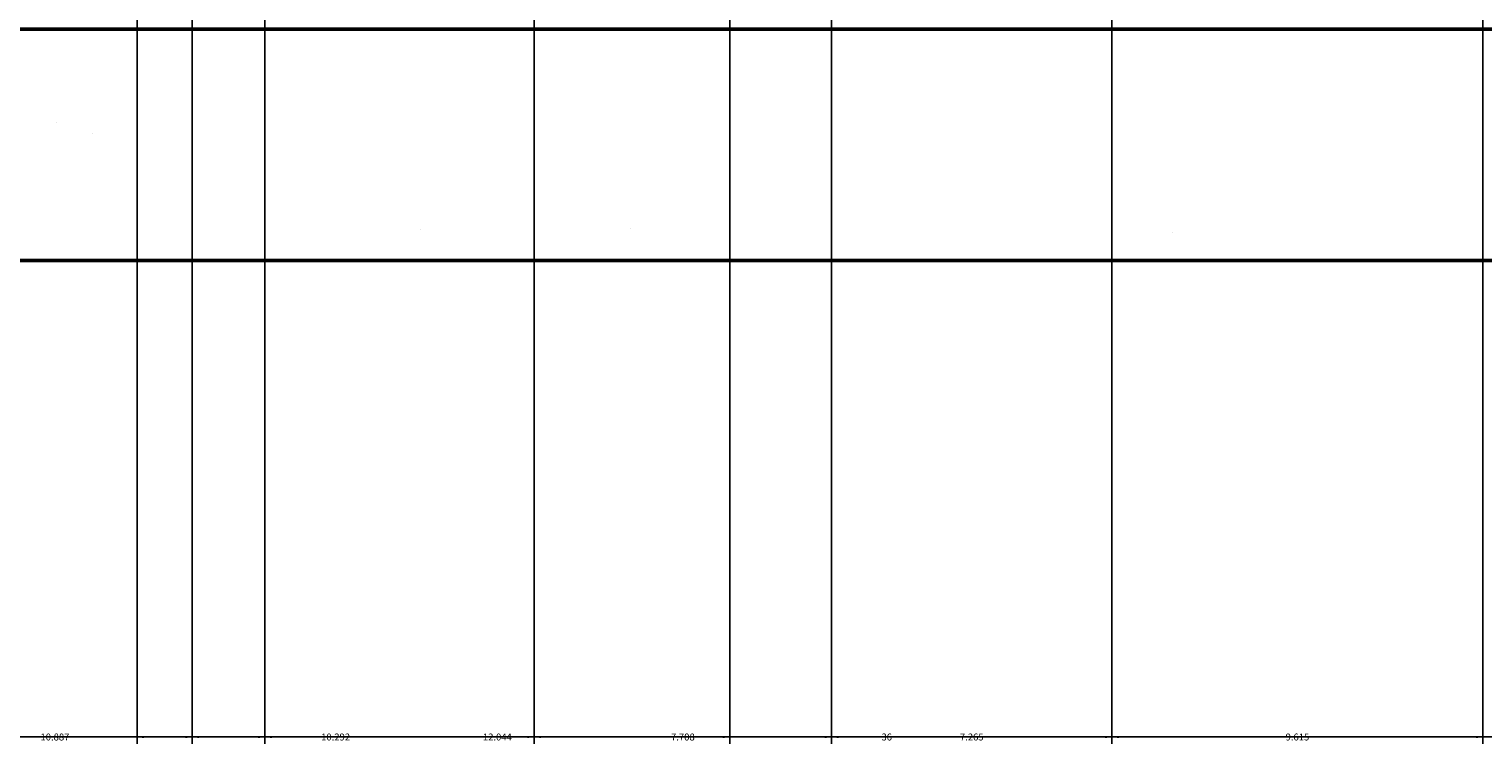
# Model space of a CAD drawing. Units: inches. Extents: x 2812 to 3051, y 1398 to 1659.
# Tile 29 of 65: x 2966 to 3004, y 1398 to 1416. Entities that reach past the tile are written whole.
import ezdxf

# ---------------------------------------------------------------- set-up
doc = ezdxf.new("R2010")
doc.units = ezdxf.units.IN
for name, color, linetype, lineweight in [('A-ANNO-DIMS', 2, 'Continuous', 18), ('S-CONC', 7, 'Continuous', 50), ('S-CONC-PATT', 8, 'Continuous', 18)]:
    doc.layers.add(name, color=color, linetype=linetype, lineweight=lineweight)
doc.styles.get("Standard").update_dxf_attribs({"font": 'arial.ttf'})
doc.dimstyles.get("Standard").update_dxf_attribs({"dimtxt": 0.18, "dimasz": 0.18, "dimexe": 0.18, "dimexo": 0.0625, "dimgap": 0.09, "dimtad": 0, "dimtih": 1, "dimtoh": 1, "dimdec": 4, "dimzin": 0, "dimdsep": 46, "dimtxsty": 'Standard', "dimcen": 0.09, "dimadec": 0, "dimazin": 0, "dimtfac": 1, "dimtdec": 4, "dimtofl": 0, "dimtmove": 0, "dimatfit": 3, "dimfxl": 1, "dimtolj": 1, "dimtzin": 0, "dimarcsym": 0})

# ---------------------------------------------------------------- blocks, each defined once
blk = doc.blocks.new('*D31')
at = {"layer": 'A-ANNO-DIMS', "color": 0, "lineweight": -2, "transparency": 16777216}
for p, q in [((2972.272, 1594.192), (2972.272, 1397.505)), ((2961.385, 1559.757), (2961.385, 1397.505)), ((2961.565, 1397.685), (2966.373, 1397.685)), ((2972.092, 1397.685), (2967.283, 1397.685))]:
    blk.add_line(p, q, dxfattribs=at)
at = {"layer": 'A-ANNO-DIMS', "color": 0, "transparency": 16777216}
for points in [[(2961.565, 1397.715), (2961.565, 1397.655), (2961.385, 1397.685)], [(2972.092, 1397.715), (2972.092, 1397.655), (2972.272, 1397.685)]]:
    blk.add_solid(points, dxfattribs=at)
at = {"layer": 'Defpoints', "color": 0, "transparency": 16777216}
for p in [(2972.272, 1594.254), (2961.385, 1559.82), (2972.272, 1397.685)]:
    blk.add_point(p, dxfattribs=at)
at = {"layer": 'A-ANNO-DIMS', "color": 0, "transparency": 16777216, "insert": (2966.828, 1397.685), "char_height": 0.18, "attachment_point": 5}
blk.add_mtext('\\A1;10.887', dxfattribs=at)
blk = doc.blocks.new('*D32')
at = {"layer": 'A-ANNO-DIMS', "color": 0, "lineweight": -2, "transparency": 16777216}
for p, q in [((2984.316, 1598.757), (2984.316, 1397.505)), ((2972.272, 1594.192), (2972.272, 1397.505)), ((2972.452, 1397.685), (2977.839, 1397.685)), ((2984.136, 1397.685), (2978.748, 1397.685))]:
    blk.add_line(p, q, dxfattribs=at)
at = {"layer": 'A-ANNO-DIMS', "color": 0, "transparency": 16777216}
for points in [[(2972.452, 1397.715), (2972.452, 1397.655), (2972.272, 1397.685)], [(2984.136, 1397.715), (2984.136, 1397.655), (2984.316, 1397.685)]]:
    blk.add_solid(points, dxfattribs=at)
at = {"layer": 'Defpoints', "color": 0, "transparency": 16777216}
for p in [(2984.316, 1598.82), (2972.272, 1594.254), (2984.316, 1397.685)]:
    blk.add_point(p, dxfattribs=at)
at = {"layer": 'A-ANNO-DIMS', "color": 0, "transparency": 16777216, "insert": (2978.294, 1397.685), "char_height": 0.18, "attachment_point": 5}
blk.add_mtext('\\A1;12.044', dxfattribs=at)
blk = doc.blocks.new('*D46')
at = {"layer": 'A-ANNO-DIMS', "color": 0, "lineweight": -2, "transparency": 16777216}
for p, q in [((2941.385, 1487.973), (2941.385, 1397.505)), ((2970.385, 1487.973), (2970.385, 1397.505)), ((2941.565, 1397.685), (2955.664, 1397.685)), ((2970.205, 1397.685), (2956.106, 1397.685))]:
    blk.add_line(p, q, dxfattribs=at)
at = {"layer": 'A-ANNO-DIMS', "color": 0, "transparency": 16777216}
for points in [[(2941.565, 1397.715), (2941.565, 1397.655), (2941.385, 1397.685)], [(2970.205, 1397.715), (2970.205, 1397.655), (2970.385, 1397.685)]]:
    blk.add_solid(points, dxfattribs=at)
at = {"layer": 'Defpoints', "color": 0, "transparency": 16777216}
for p in [(2941.385, 1488.035), (2970.385, 1488.035), (2970.385, 1397.685)]:
    blk.add_point(p, dxfattribs=at)
at = {"layer": 'A-ANNO-DIMS', "color": 0, "transparency": 16777216, "insert": (2955.885, 1397.685), "char_height": 0.18, "attachment_point": 5}
blk.add_mtext('\\A1;29', dxfattribs=at)
blk = doc.blocks.new('*D47')
at = {"layer": 'A-ANNO-DIMS', "color": 0, "lineweight": -2, "transparency": 16777216}
for p, q in [((2970.385, 1487.973), (2970.385, 1397.505)), ((3006.385, 1487.973), (3006.385, 1397.505)), ((2970.565, 1397.685), (2988.166, 1397.685)), ((3006.205, 1397.685), (2988.604, 1397.685))]:
    blk.add_line(p, q, dxfattribs=at)
at = {"layer": 'A-ANNO-DIMS', "color": 0, "transparency": 16777216}
for points in [[(2970.565, 1397.715), (2970.565, 1397.655), (2970.385, 1397.685)], [(3006.205, 1397.715), (3006.205, 1397.655), (3006.385, 1397.685)]]:
    blk.add_solid(points, dxfattribs=at)
at = {"layer": 'Defpoints', "color": 0, "transparency": 16777216}
for p in [(2970.385, 1488.035), (3006.385, 1488.035), (3006.385, 1397.685)]:
    blk.add_point(p, dxfattribs=at)
at = {"layer": 'A-ANNO-DIMS', "color": 0, "transparency": 16777216, "insert": (2988.385, 1397.685), "char_height": 0.18, "attachment_point": 5}
blk.add_mtext('\\A1;36', dxfattribs=at)
blk = doc.blocks.new('*D71')
at = {"layer": 'A-ANNO-DIMS', "color": 0, "lineweight": -2, "transparency": 16777216}
for p, q in [((2968.956, 1466.685), (2968.956, 1397.505)), ((2979.248, 1456.685), (2979.248, 1397.505)), ((2969.136, 1397.685), (2973.648, 1397.685)), ((2979.068, 1397.685), (2974.556, 1397.685))]:
    blk.add_line(p, q, dxfattribs=at)
at = {"layer": 'A-ANNO-DIMS', "color": 0, "transparency": 16777216}
for points in [[(2969.136, 1397.715), (2969.136, 1397.655), (2968.956, 1397.685)], [(2979.068, 1397.715), (2979.068, 1397.655), (2979.248, 1397.685)]]:
    blk.add_solid(points, dxfattribs=at)
at = {"layer": 'Defpoints', "color": 0, "transparency": 16777216}
for p in [(2968.956, 1466.747), (2979.248, 1456.747), (2979.248, 1397.685)]:
    blk.add_point(p, dxfattribs=at)
at = {"layer": 'A-ANNO-DIMS', "color": 0, "transparency": 16777216, "insert": (2974.102, 1397.685), "char_height": 0.18, "attachment_point": 5}
blk.add_mtext('\\A1;10.292', dxfattribs=at)
blk = doc.blocks.new('*D72')
at = {"layer": 'A-ANNO-DIMS', "color": 0, "lineweight": -2, "transparency": 16777216}
for p, q in [((2979.248, 1456.685), (2979.248, 1397.505)), ((2986.956, 1446.685), (2986.956, 1397.505)), ((2979.428, 1397.685), (2982.709, 1397.685)), ((2986.776, 1397.685), (2983.495, 1397.685))]:
    blk.add_line(p, q, dxfattribs=at)
at = {"layer": 'A-ANNO-DIMS', "color": 0, "transparency": 16777216}
for points in [[(2979.428, 1397.715), (2979.428, 1397.655), (2979.248, 1397.685)], [(2986.776, 1397.715), (2986.776, 1397.655), (2986.956, 1397.685)]]:
    blk.add_solid(points, dxfattribs=at)
at = {"layer": 'Defpoints', "color": 0, "transparency": 16777216}
for p in [(2979.248, 1456.747), (2986.956, 1446.747), (2986.956, 1397.685)]:
    blk.add_point(p, dxfattribs=at)
at = {"layer": 'A-ANNO-DIMS', "color": 0, "transparency": 16777216, "insert": (2983.102, 1397.685), "char_height": 0.18, "attachment_point": 5}
blk.add_mtext('\\A1;7.708', dxfattribs=at)
blk = doc.blocks.new('*D73')
at = {"layer": 'A-ANNO-DIMS', "color": 0, "lineweight": -2, "transparency": 16777216}
for p, q in [((2986.956, 1446.685), (2986.956, 1397.505)), ((2994.221, 1436.685), (2994.221, 1397.505)), ((2987.136, 1397.685), (2990.195, 1397.685)), ((2994.041, 1397.685), (2990.982, 1397.685))]:
    blk.add_line(p, q, dxfattribs=at)
at = {"layer": 'A-ANNO-DIMS', "color": 0, "transparency": 16777216}
for points in [[(2987.136, 1397.715), (2987.136, 1397.655), (2986.956, 1397.685)], [(2994.041, 1397.715), (2994.041, 1397.655), (2994.221, 1397.685)]]:
    blk.add_solid(points, dxfattribs=at)
at = {"layer": 'Defpoints', "color": 0, "transparency": 16777216}
for p in [(2986.956, 1446.747), (2994.221, 1436.747), (2994.221, 1397.685)]:
    blk.add_point(p, dxfattribs=at)
at = {"layer": 'A-ANNO-DIMS', "color": 0, "transparency": 16777216, "insert": (2990.589, 1397.685), "char_height": 0.18, "attachment_point": 5}
blk.add_mtext('\\A1;7.265', dxfattribs=at)
blk = doc.blocks.new('*D74')
at = {"layer": 'A-ANNO-DIMS', "color": 0, "lineweight": -2, "transparency": 16777216}
for p, q in [((2994.221, 1436.685), (2994.221, 1397.505)), ((3003.837, 1426.685), (3003.837, 1397.505)), ((2994.401, 1397.685), (2998.635, 1397.685)), ((3003.657, 1397.685), (2999.423, 1397.685))]:
    blk.add_line(p, q, dxfattribs=at)
at = {"layer": 'A-ANNO-DIMS', "color": 0, "transparency": 16777216}
for points in [[(2994.401, 1397.715), (2994.401, 1397.655), (2994.221, 1397.685)], [(3003.657, 1397.715), (3003.657, 1397.655), (3003.837, 1397.685)]]:
    blk.add_solid(points, dxfattribs=at)
at = {"layer": 'Defpoints', "color": 0, "transparency": 16777216}
for p in [(2994.221, 1436.747), (3003.837, 1426.747), (3003.837, 1397.685)]:
    blk.add_point(p, dxfattribs=at)
at = {"layer": 'A-ANNO-DIMS', "color": 0, "transparency": 16777216, "insert": (2999.029, 1397.685), "char_height": 0.18, "attachment_point": 5}
blk.add_mtext('\\A1;9.615', dxfattribs=at)

msp = doc.modelspace()

# ---------------------------------------------------------------- hatches: boundary and pattern name
at = {"layer": 'S-CONC-PATT'}
h = msp.add_hatch(dxfattribs=at)
h.set_pattern_fill('AR-SAND', color=256, scale=0.3)
h.paths.add_polyline_path([(3036.3849, 1416.0354), (3027.3849, 1416.0354), (2826.3849, 1416.0354), (2826.3849, 1410.0354), (2835.3849, 1410.0354), (3036.3849, 1410.0354)])
h.paths.add_polyline_path([(2970.3849, 1488.0354), (2969.3849, 1488.0354), (2941.3849, 1488.0354), (2941.3849, 1482.0354), (2970.3849, 1482.0354)])
h.paths.add_polyline_path([(3036.3849, 1488.0354), (3035.3849, 1488.0354), (3006.3849, 1488.0354), (3006.3849, 1482.0354), (3027.3849, 1482.0354), (3036.3849, 1482.0354)])
h.paths.add_polyline_path([(3034.3849, 1490.0354), (3008.3849, 1490.0354), (3008.3849, 1489.0354), (3034.3849, 1489.0354)])
h.paths.add_polyline_path([(3035.3849, 1489.0354), (3034.3849, 1489.0354), (3007.3849, 1489.0354), (3007.3849, 1488.0354), (3035.3849, 1488.0354)])
h.paths.add_polyline_path([(2968.3849, 1490.0354), (2943.3849, 1490.0354), (2943.3849, 1489.0354), (2968.3849, 1489.0354)])
h.paths.add_polyline_path([(2969.3849, 1489.0354), (2968.3849, 1489.0354), (2942.3849, 1489.0354), (2942.3849, 1488.0354), (2969.3849, 1488.0354)])
h.paths.add_polyline_path([(2896.3849, 1488.0354), (2826.3849, 1488.0354), (2826.3849, 1482.0354), (2896.3849, 1482.0354)])
h.paths.add_polyline_path([(2895.3849, 1489.0354), (2894.3849, 1489.0354), (2827.3849, 1489.0354), (2827.3849, 1488.0354), (2895.3849, 1488.0354)])
h.paths.add_polyline_path([(2894.3849, 1490.0354), (2828.3849, 1490.0354), (2828.3849, 1489.0354), (2894.3849, 1489.0354)])
h = msp.add_hatch(dxfattribs=at)
h.set_pattern_fill('AR-CONC', color=256, scale=0.3)
h.paths.add_polyline_path([(3036.3849, 1416.0354), (3027.3849, 1416.0354), (2826.3849, 1416.0354), (2826.3849, 1410.0354), (2835.3849, 1410.0354), (3036.3849, 1410.0354)])

# ---------------------------------------------------------------- linework, layer by layer
at = {"layer": 'S-CONC'}
for p, q in [((2826.3849, 1416.0354), (3027.3849, 1416.0354)), ((2835.3849, 1410.0354), (3036.3849, 1410.0354))]:
    msp.add_line(p, q, dxfattribs=at)

# ---------------------------------------------------------------- dimensions: what is measured, and where the dimension line sits
at = {"layer": 'A-ANNO-DIMS'}
for base, p1, p2, override, picture, middle in [((2984.3156, 1397.6854), (2972.2716, 1594.2541), (2984.3156, 1598.82), {"dimdec": 3, "dimlfac": 1, "dimrnd": 0, "dimzin": 0, "dimdsep": 46, "dimlunit": 2}, '*D32', (2978.2936, 1397.6854)), ((2972.2716, 1397.6854), (2961.3849, 1559.82), (2972.2716, 1594.2541), {"dimdec": 3, "dimlfac": 1, "dimrnd": 0, "dimzin": 0, "dimdsep": 46, "dimlunit": 2}, '*D31', (2966.8282, 1397.6854)), ((2970.3849, 1397.6854), (2941.3849, 1488.0354), (2970.3849, 1488.0354), {"dimdec": 0, "dimlfac": 1, "dimrnd": 0, "dimzin": 0, "dimdsep": 46, "dimlunit": 2}, '*D46', (2955.8849, 1397.6854)), ((3006.3849, 1397.6854), (2970.3849, 1488.0354), (3006.3849, 1488.0354), {"dimdec": 0, "dimlfac": 1, "dimrnd": 0, "dimzin": 0, "dimdsep": 46, "dimlunit": 2}, '*D47', (2988.3849, 1397.6854)), ((2979.2478, 1397.6854), (2968.9558, 1466.7474), (2979.2478, 1456.7474), {"dimdec": 3, "dimlfac": 1, "dimrnd": 0, "dimzin": 0, "dimdsep": 46, "dimlunit": 2}, '*D71', (2974.1018, 1397.6854)), ((2986.9558, 1397.6854), (2979.2478, 1456.7474), (2986.9558, 1446.7474), {"dimdec": 3, "dimlfac": 1, "dimrnd": 0, "dimzin": 0, "dimdsep": 46, "dimlunit": 2}, '*D72', (2983.1018, 1397.6854)), ((2994.22128, 1397.6854), (2986.95585, 1446.74738), (2994.22128, 1436.74738), {"dimdec": 3, "dimlfac": 1, "dimrnd": 0, "dimzin": 0, "dimdsep": 46, "dimlunit": 2}, '*D73', (2990.58856, 1397.6854)), ((3003.83676, 1397.6854), (2994.22128, 1436.74738), (3003.83676, 1426.74738), {"dimdec": 3, "dimlfac": 1, "dimrnd": 0, "dimzin": 0, "dimdsep": 46, "dimlunit": 2}, '*D74', (2999.02902, 1397.6854))]:
    dim = msp.add_linear_dim(base=base, p1=p1, p2=p2, dimstyle='Standard', override=override, dxfattribs=at)
    dim.commit()
    dim.dimension.update_dxf_attribs({"geometry": picture, "text_midpoint": middle})

doc.saveas('drawing.dxf')
